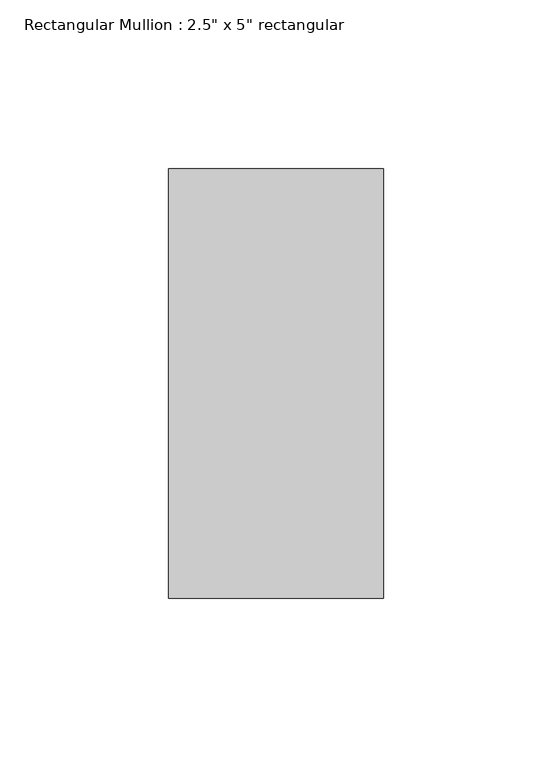
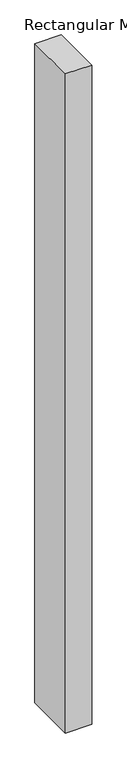
"""IFC4 building model written with IfcOpenShell, lengths in millimetres: member geometry."""

from ifc_helpers import new_model, si_unit, frame, origin, place, context, project, spatial, polyline, outline, extrude, source, transform, mapped, element, save


def member_3b0b484b(model_context):
    return source(origin(), model_context, "Body", "SweptSolid", [
        extrude(outline(polyline([(31.75, 63.5), (31.75, -63.5), (-31.75, -63.5), (-31.75, 63.5), (31.75, 63.5)])), frame((0.0, 0.0, -1675.41517), z_axis=(0.0, 0.0, 1.0), x_axis=(1.0, 0.0, 0.0)), (0.0, 0.0, 1.0), 1675.41517),
    ])


if __name__ == "__main__":
    model = new_model("IFC4")
    model_context = context("Model", 3, world=origin())
    ifc_project = project(units=[si_unit("LENGTHUNIT", "METRE", prefix="MILLI")], contexts=[model_context])
    site = spatial("IfcSite", under=ifc_project)
    building = spatial("IfcBuilding", under=site)
    placement = place(None, origin())
    member_shape = member_3b0b484b(model_context)
    element("IfcMember", 1, ObjectType="Rectangular Mullion : 2.5\" x 5\" rectangular", at=placement, inside=building, context=model_context, shape_type="MappedRepresentation", body=[
        mapped(member_shape, transform((0.0, 0.0, 0.0), x_axis=(1.0, 0.0, 0.0), y_axis=(0.0, 1.0, 0.0), z_axis=(0.0, 0.0, 1.0))),
    ])
    save(model, "model.ifc")

# Revit data of these elements
# Type "Rectangular Mullion : 2.5\" x 5\" rectangular"
#   built-in parameter 1007304 = 0.416667 (stored number, unit not read)
#   built-in parameter 1007301 = 0.104167 (stored number, unit not read)
#   built-in parameter 1007300 = 0.104167 (stored number, unit not read)
# Element 1 (IfcMember, "Rectangular Mullion : 2.5\" x 5\" rectangular")
#   Materials on its faces: "Aluminum"
# Materials
#   "Aluminum": class "Metal", colour RGB 247 247 247, transparency 0, Description = "Aluminum 6061", Cost = 0
